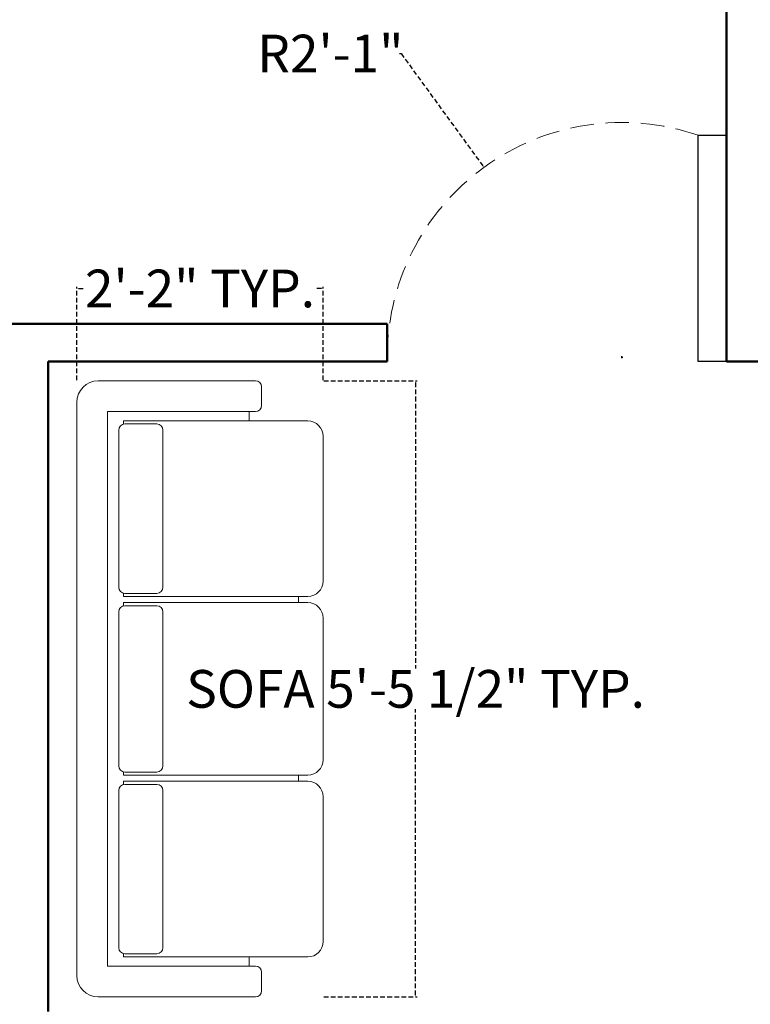
# Model space of a CAD drawing. Units: inches. Extents: x 513 to 1142, y 396 to 927.
# Tile 5 of 31: x 665 to 743, y 642 to 746. Entities that reach past the tile are written whole.
import ezdxf

# ---------------------------------------------------------------- set-up
doc = ezdxf.new("R2010")
doc.units = ezdxf.units.IN
doc.header["$MEASUREMENT"] = 0
doc.linetypes.add('DASHED', pattern=[0.75, 0.5, -0.25])
for name, color, linetype, lineweight in [('A-ANNO-DIMS', 2, 'DASHED', 18), ('A-DOOR', 4, 'Continuous', 25), ('A-DOOR-SWNG', 4, 'DASHED', 13), ('A-WALL', 7, 'Continuous', 50), ('furniture', 92, 'Continuous', 18)]:
    doc.layers.add(name, color=color, linetype=linetype, lineweight=lineweight)
doc.styles.get("Standard").update_dxf_attribs({"font": 'arial.ttf'})
doc.dimstyles.get("Standard").update_dxf_attribs({"dimtxt": 4, "dimasz": 0.18, "dimexe": 0.18, "dimexo": 0.0625, "dimgap": 0.09, "dimtad": 0, "dimtih": 1, "dimtoh": 1, "dimdec": 0, "dimrnd": 6, "dimzin": 0, "dimdsep": 46, "dimlunit": 3, "dimtxsty": 'Standard', "dimcen": 0.09, "dimadec": 0, "dimazin": 0, "dimtfac": 1, "dimtdec": 0, "dimtofl": 0, "dimtmove": 0, "dimatfit": 3, "dimfxl": 1, "dimtolj": 1, "dimtzin": 0, "dimarcsym": 0})

# ---------------------------------------------------------------- blocks, each defined once
blk = doc.blocks.new('A$C06FC73D7')
for p, q in [((1.93, 0.8), (0.07, 0.8)), ((0, 0.73), (0, 0.22)), ((2, 0.22), (2, 0.73)), ((0.1, 0.22), (0.1, 0.7)), ((0.1, 0.7), (1.9, 0.7)), ((1.9, 0.7), (1.9, 0.22)), ((0.13, 0.6479), (0.13, 0.05)), ((0.1404, 0.6479), (0.13, 0.6479)), ((0.14, 0.54), (0.14, 0.6437)), ((0.67, 0.6637), (0.16, 0.6637)), ((0.7, 0.6479), (0.6896, 0.6479)), ((0.69, 0.54), (0.69, 0.6437)), ((0.7, 0.05), (0.7, 0.6479)), ((0.72, 0.05), (0.72, 0.6479)), ((0.7304, 0.6479), (0.72, 0.6479)), ((0.73, 0.54), (0.73, 0.6437)), ((1.25, 0.6637), (0.75, 0.6637)), ((1.28, 0.6479), (1.2696, 0.6479)), ((1.27, 0.54), (1.27, 0.6437)), ((1.28, 0.05), (1.28, 0.6479)), ((1.3, 0.05), (1.3, 0.6479)), ((1.3104, 0.6479), (1.3, 0.6479)), ((1.31, 0.54), (1.31, 0.6437)), ((1.84, 0.6637), (1.33, 0.6637)), ((1.87, 0.6479), (1.86, 0.6479)), ((1.86, 0.54), (1.86, 0.6437)), ((1.87, 0.05), (1.87, 0.6479)), ((0.67, 0.52), (0.16, 0.52)), ((1.25, 0.52), (0.75, 0.52)), ((1.84, 0.52), (1.33, 0.52)), ((0.13, 0.24), (0.1, 0.24)), ((1.9, 0.24), (1.87, 0.24)), ((0.02, 0.2), (0.08, 0.2)), ((1.92, 0.2), (1.98, 0.2)), ((0.72, 0.08), (0.7, 0.08)), ((1.3, 0.08), (1.28, 0.08)), ((0.65, 0), (0.18, 0)), ((1.23, 0), (0.77, 0)), ((1.82, 0), (1.35, 0))]:
    blk.add_line(p, q)
for centre, radius, start, end in [((0.07, 0.73), 0.07, 90, 180), ((1.93, 0.73), 0.07, 0, 90), ((0.16, 0.6437), 0.02, 90, 180), ((0.67, 0.6437), 0.02, 0, 90), ((0.75, 0.6437), 0.02, 90, 180), ((1.25, 0.6437), 0.02, 0, 90), ((1.33, 0.6437), 0.02, 90, 180), ((1.84, 0.6437), 0.02, 0, 90), ((0.16, 0.54), 0.02, 180, 270), ((0.67, 0.54), 0.02, 270, 0), ((0.75, 0.54), 0.02, 180, 270), ((1.25, 0.54), 0.02, 270, 0), ((1.33, 0.54), 0.02, 180, 270), ((1.84, 0.54), 0.02, 270, 0), ((0.02, 0.22), 0.02, 180, 270), ((0.08, 0.22), 0.02, 270, 0), ((1.92, 0.22), 0.02, 180, 270), ((1.98, 0.22), 0.02, 270, 0), ((0.18, 0.05), 0.05, 180, 270), ((0.65, 0.05), 0.05, 270, 0), ((0.77, 0.05), 0.05, 180, 270), ((1.23, 0.05), 0.05, 270, 0), ((1.35, 0.05), 0.05, 180, 270), ((1.82, 0.05), 0.05, 270, 0)]:
    blk.add_arc(centre, radius, start, end)
blk = doc.blocks.new('A$C2BDD4447')
blk.add_blockref('A$C06FC73D7', (0, 0))
blk = doc.blocks.new('DOOR-LEAF-24IN')
blk.add_lwpolyline([(3, 24), (3, 0), (0, 0), (0, 24)], close=True)
blk = doc.blocks.new('*D119')
at = {"layer": 'A-ANNO-DIMS', "color": 0, "lineweight": -2, "transparency": 16777216}
for p, q in [((697.25, 708.1), (707.18, 708.1)), ((707, 707.92), (707, 677.57)), ((707, 642.9), (707, 673.25)), ((697.25, 642.72), (707.18, 642.72))]:
    blk.add_line(p, q, dxfattribs=at)
at = {"layer": 'A-ANNO-DIMS', "color": 0, "transparency": 16777216}
for points in [[(706.97, 707.92), (707.03, 707.92), (707, 708.1)], [(706.97, 642.9), (707.03, 642.9), (707, 642.72)]]:
    blk.add_solid(points, dxfattribs=at)
at = {"layer": 'Defpoints', "color": 0, "transparency": 16777216}
for p in [(697.19, 708.1), (707, 708.1), (697.19, 642.72)]:
    blk.add_point(p, dxfattribs=at)
at = {"layer": 'A-ANNO-DIMS', "color": 0, "transparency": 16777216, "insert": (707, 675.41), "char_height": 4, "attachment_point": 5}
blk.add_mtext('\\A1;SOFA 5\'-5 1/2" TYP.', dxfattribs=at)
blk = doc.blocks.new('*D120')
at = {"layer": 'A-ANNO-DIMS', "color": 0, "lineweight": -2, "transparency": 16777216}
for p, q in [((671.04, 708.16), (671.04, 718.08)), ((671.22, 717.9), (671.8, 717.9)), ((697.01, 717.9), (696.43, 717.9)), ((697.19, 708.16), (697.19, 718.08))]:
    blk.add_line(p, q, dxfattribs=at)
at = {"layer": 'A-ANNO-DIMS', "color": 0, "transparency": 16777216}
for points in [[(671.22, 717.93), (671.22, 717.87), (671.04, 717.9)], [(697.01, 717.93), (697.01, 717.87), (697.19, 717.9)]]:
    blk.add_solid(points, dxfattribs=at)
at = {"layer": 'Defpoints', "color": 0, "transparency": 16777216}
for p in [(671.04, 717.9), (671.04, 708.1), (697.19, 708.1)]:
    blk.add_point(p, dxfattribs=at)
at = {"layer": 'A-ANNO-DIMS', "color": 0, "transparency": 16777216, "insert": (684.12, 717.9), "char_height": 4, "attachment_point": 5}
blk.add_mtext('\\A1;2\'-2" TYP.', dxfattribs=at)
blk = doc.blocks.new('*D183')
at = {"layer": 'A-ANNO-DIMS', "color": 0, "lineweight": -2, "transparency": 16777216}
for p, q in [((705.28, 742.83), (705.46, 742.83)), ((705.46, 742.83), (714.14, 730.9)), ((728.8, 710.61), (728.98, 710.61)), ((728.89, 710.52), (728.89, 710.7))]:
    blk.add_line(p, q, dxfattribs=at)
at = {"layer": 'A-ANNO-DIMS', "color": 0, "transparency": 16777216}
blk.add_solid([(714.16, 730.92), (714.12, 730.88), (714.25, 730.75)], dxfattribs=at)
at = {"layer": 'Defpoints', "color": 0, "transparency": 16777216}
for p in [(714.25, 730.75), (728.89, 710.61)]:
    blk.add_point(p, dxfattribs=at)
at = {"layer": 'A-ANNO-DIMS', "color": 0, "transparency": 16777216, "insert": (697.96, 742.83), "char_height": 4, "attachment_point": 5}
blk.add_mtext('\\A1;R2\'-1"', dxfattribs=at)

msp = doc.modelspace()

# ---------------------------------------------------------------- linework, layer by layer
at = {"layer": 'A-DOOR-SWNG', "ltscale": 5}
msp.add_arc((728.89, 710.61), 24.9, 71.005, 181.0498, dxfattribs=at)
at = {"layer": 'A-WALL'}
for p, q in [((740, 870.16), (740, 710.16)), ((704, 714.16), (664, 714.16)), ((704, 714.16), (704, 710.16)), ((704, 710.16), (668, 710.16)), ((668, 710.16), (668, 641.16)), ((744, 710.16), (740, 710.16))]:
    msp.add_line(p, q, dxfattribs=at)

# ---------------------------------------------------------------- block references
at = {"layer": 'A-DOOR'}
msp.add_blockref('DOOR-LEAF-24IN', (736.99, 710.16), dxfattribs=at)
at = {"layer": 'furniture', "xscale": 32.68979708061804, "yscale": 32.68979708061804, "zscale": 32.68979708061804, "rotation": 90}
msp.add_blockref('A$C2BDD4447', (697.19, 642.72), dxfattribs=at)

# ---------------------------------------------------------------- dimensions: what is measured, and where the dimension line sits
at = {"layer": 'A-ANNO-DIMS'}
dim = msp.add_radius_dim(center=(728.89, 710.61), mpoint=(714.25, 730.75), dimstyle='Standard', override={"dimdec": 1, "dimlfac": 1, "dimrnd": 0, "dimzin": 1, "dimdsep": 46, "dimlunit": 4, "dimfrac": 2}, dxfattribs=at)
dim.commit()
dim.dimension.update_dxf_attribs({"geometry": '*D183', "text_midpoint": (697.96, 742.83), "dimtype": 164})
for base, p1, p2, angle, text, picture, middle in [((671.0403, 717.9023), (697.1921, 708.0953), (671.0403, 708.0953), 180, '<> TYP.', '*D120', (684.1162, 717.9023)), ((707, 708.1), (697.19, 642.72), (697.19, 708.1), 90, 'SOFA <> TYP.', '*D119', (707, 675.41))]:
    dim = msp.add_linear_dim(base=base, p1=p1, p2=p2, angle=angle, text=text, dimstyle='Standard', override={"dimdec": 1, "dimlfac": 1, "dimrnd": 0, "dimzin": 1, "dimdsep": 46, "dimlunit": 4, "dimfrac": 2}, dxfattribs=at)
    dim.commit()
    dim.dimension.update_dxf_attribs({"geometry": picture, "text_midpoint": middle})

doc.saveas('drawing.dxf')
